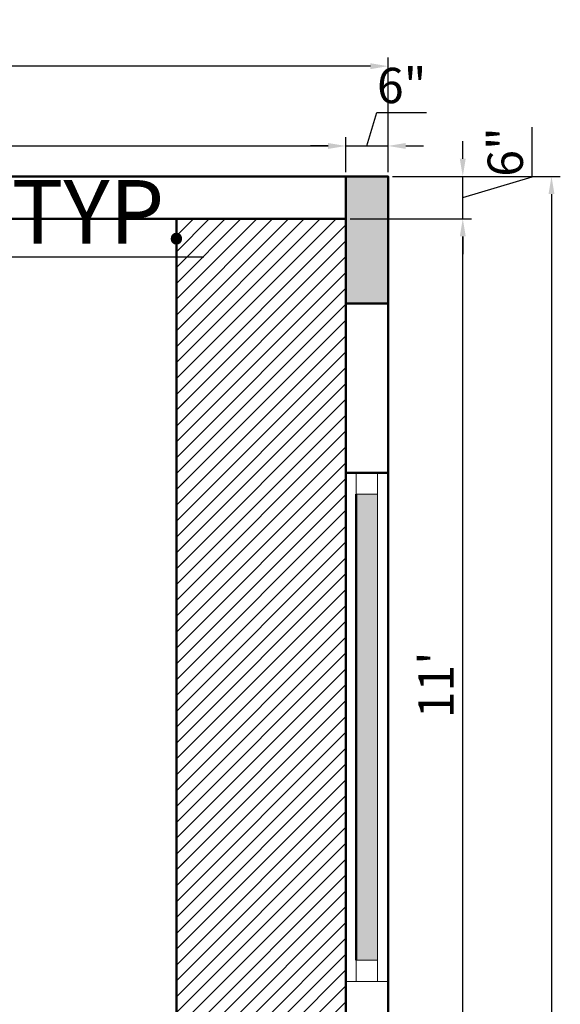
# Model space of a CAD drawing. Units: inches. Extents: x 3064 to 19385, y 846 to 15425.
# Tile 48 of 108: x 5481 to 5557, y 1275 to 1414. Entities that reach past the tile are written whole.
import ezdxf

# ---------------------------------------------------------------- set-up
doc = ezdxf.new("R2010")
doc.units = ezdxf.units.IN
for name, color, linetype, lineweight in [('A-ANNO-DIMS', 2, 'Continuous', 18), ('A-COLS', 1, 'Continuous', 35), ('A-FURN-PATT', 252, 'Continuous', 13), ('A-GLAZ', 4, 'Continuous', 18), ('A-WALL', 7, 'Continuous', 50)]:
    doc.layers.add(name, color=color, linetype=linetype, lineweight=lineweight)
doc.styles.get("Standard").update_dxf_attribs({"font": 'arial.ttf'})
doc.dimstyles.new('ISO-25', dxfattribs={"dimtxt": 9, "dimasz": 2.5, "dimexe": 1.25, "dimexo": 0.625, "dimtad": 1, "dimdec": 1, "dimlunit": 3, "dimtxsty": 'Standard', "dimcen": 2.5, "dimadec": 0, "dimazin": 0, "dimtfac": 1, "dimtdec": 1, "dimtmove": 0, "dimatfit": 3, "dimfxl": 1, "dimarcsym": 0})

# ---------------------------------------------------------------- blocks, each defined once
blk = doc.blocks.new('*D86')
at = {"layer": 'A-ANNO-DIMS', "color": 0, "lineweight": -2, "transparency": 16777216}
for p, q in [((5527.64, 1386.1), (5544.85, 1386.1)), ((5543.6, 1256.6), (5543.6, 1383.6)), ((5533.64, 1254.1), (5544.85, 1254.1))]:
    blk.add_line(p, q, dxfattribs=at)
at = {"layer": 'A-ANNO-DIMS', "color": 0, "transparency": 16777216}
for points in [[(5543.18, 1383.6), (5544.02, 1383.6), (5543.6, 1386.1)], [(5543.18, 1256.6), (5544.02, 1256.6), (5543.6, 1254.1)]]:
    blk.add_solid(points, dxfattribs=at)
at = {"layer": 'Defpoints', "color": 0, "transparency": 16777216}
for p in [(5527.02, 1386.1), (5543.6, 1386.1), (5533.02, 1254.1)]:
    blk.add_point(p, dxfattribs=at)
at = {"layer": 'A-ANNO-DIMS', "color": 0, "transparency": 16777216, "insert": (5540.46, 1320.1), "char_height": 5, "attachment_point": 5, "rotation": 90}
blk.add_mtext("11'", dxfattribs=at)
blk = doc.blocks.new('*D87')
at = {"layer": 'A-ANNO-DIMS', "color": 0, "lineweight": -2, "transparency": 16777216}
for p, q in [((5553.45, 1392.05), (5553.45, 1399.07)), ((5543.6, 1394.6), (5543.6, 1397.1)), ((5533.64, 1392.1), (5544.85, 1392.1)), ((5543.6, 1386.1), (5543.6, 1392.1)), ((5543.6, 1386.1), (5543.6, 1392.1)), ((5543.6, 1389.1), (5553.45, 1392.05)), ((5527.64, 1386.1), (5544.85, 1386.1)), ((5543.6, 1383.6), (5543.6, 1381.1))]:
    blk.add_line(p, q, dxfattribs=at)
at = {"layer": 'A-ANNO-DIMS', "color": 0, "transparency": 16777216}
for points in [[(5543.18, 1394.6), (5544.02, 1394.6), (5543.6, 1392.1)], [(5543.18, 1383.6), (5544.02, 1383.6), (5543.6, 1386.1)]]:
    blk.add_solid(points, dxfattribs=at)
at = {"layer": 'Defpoints', "color": 0, "transparency": 16777216}
for p in [(5533.02, 1392.1), (5543.6, 1392.1), (5527.02, 1386.1)]:
    blk.add_point(p, dxfattribs=at)
at = {"layer": 'A-ANNO-DIMS', "color": 0, "transparency": 16777216, "insert": (5550.27, 1395.56), "char_height": 5, "attachment_point": 5, "rotation": 90}
blk.add_mtext('6"', dxfattribs=at)
blk = doc.blocks.new('*D88')
at = {"layer": 'A-ANNO-DIMS', "color": 0, "lineweight": -2, "transparency": 16777216}
for p, q in [((5533.64, 1392.1), (5557.42, 1392.1)), ((5556.17, 1389.6), (5556.17, 902.6)), ((5533.64, 900.1), (5557.42, 900.1))]:
    blk.add_line(p, q, dxfattribs=at)
at = {"layer": 'A-ANNO-DIMS', "color": 0, "transparency": 16777216}
for points in [[(5555.75, 1389.6), (5556.59, 1389.6), (5556.17, 1392.1)], [(5555.75, 902.6), (5556.59, 902.6), (5556.17, 900.1)]]:
    blk.add_solid(points, dxfattribs=at)
at = {"layer": 'Defpoints', "color": 0, "transparency": 16777216}
for p in [(5533.02, 1392.1), (5533.02, 900.1), (5556.17, 900.1)]:
    blk.add_point(p, dxfattribs=at)
at = {"layer": 'A-ANNO-DIMS', "color": 0, "transparency": 16777216, "insert": (5553.04, 1146.1), "char_height": 5, "attachment_point": 5, "rotation": 90}
blk.add_mtext("41'", dxfattribs=at)
blk = doc.blocks.new('*D92')
at = {"layer": 'A-ANNO-DIMS', "color": 0, "lineweight": -2, "transparency": 16777216}
for p, q in [((5332.02, 1392.72), (5332.02, 1397.66)), ((5527.02, 1392.72), (5527.02, 1397.66)), ((5334.52, 1396.41), (5524.52, 1396.41))]:
    blk.add_line(p, q, dxfattribs=at)
at = {"layer": 'A-ANNO-DIMS', "color": 0, "transparency": 16777216}
for points in [[(5334.52, 1396.83), (5334.52, 1395.99), (5332.02, 1396.41)], [(5524.52, 1396.83), (5524.52, 1395.99), (5527.02, 1396.41)]]:
    blk.add_solid(points, dxfattribs=at)
at = {"layer": 'Defpoints', "color": 0, "transparency": 16777216}
for p in [(5527.02, 1396.41), (5332.02, 1392.1), (5527.02, 1392.1)]:
    blk.add_point(p, dxfattribs=at)
at = {"layer": 'A-ANNO-DIMS', "color": 0, "transparency": 16777216, "insert": (5429.52, 1399.59), "char_height": 5, "attachment_point": 5}
blk.add_mtext('16\'-3"', dxfattribs=at)
blk = doc.blocks.new('*D93')
at = {"layer": 'A-ANNO-DIMS', "color": 0, "lineweight": -2, "transparency": 16777216}
for p, q in [((5530.02, 1396.41), (5531.44, 1401.15)), ((5531.44, 1401.15), (5538.46, 1401.15)), ((5527.02, 1392.72), (5527.02, 1397.66)), ((5533.02, 1392.72), (5533.02, 1397.66)), ((5524.52, 1396.41), (5522.02, 1396.41)), ((5527.02, 1396.41), (5533.02, 1396.41)), ((5527.02, 1396.41), (5533.02, 1396.41)), ((5535.52, 1396.41), (5538.02, 1396.41))]:
    blk.add_line(p, q, dxfattribs=at)
at = {"layer": 'A-ANNO-DIMS', "color": 0, "transparency": 16777216}
for points in [[(5524.52, 1396.83), (5524.52, 1395.99), (5527.02, 1396.41)], [(5535.52, 1396.83), (5535.52, 1395.99), (5533.02, 1396.41)]]:
    blk.add_solid(points, dxfattribs=at)
at = {"layer": 'Defpoints', "color": 0, "transparency": 16777216}
for p in [(5533.02, 1396.41), (5527.02, 1392.1), (5533.02, 1392.1)]:
    blk.add_point(p, dxfattribs=at)
at = {"layer": 'A-ANNO-DIMS', "color": 0, "transparency": 16777216, "insert": (5534.95, 1404.33), "char_height": 5, "attachment_point": 5}
blk.add_mtext('6"', dxfattribs=at)
blk = doc.blocks.new('*D94')
at = {"layer": 'A-ANNO-DIMS', "color": 0, "lineweight": -2, "transparency": 16777216}
for p, q in [((5191.02, 1392.72), (5191.02, 1408.96)), ((5533.02, 1392.72), (5533.02, 1408.96)), ((5530.52, 1407.71), (5193.52, 1407.71))]:
    blk.add_line(p, q, dxfattribs=at)
at = {"layer": 'A-ANNO-DIMS', "color": 0, "transparency": 16777216}
for points in [[(5193.52, 1408.12), (5193.52, 1407.29), (5191.02, 1407.71)], [(5530.52, 1408.12), (5530.52, 1407.29), (5533.02, 1407.71)]]:
    blk.add_solid(points, dxfattribs=at)
at = {"layer": 'Defpoints', "color": 0, "transparency": 16777216}
for p in [(5191.02, 1407.71), (5191.02, 1392.1), (5533.02, 1392.1)]:
    blk.add_point(p, dxfattribs=at)
at = {"layer": 'A-ANNO-DIMS', "color": 0, "transparency": 16777216, "insert": (5362.02, 1410.88), "char_height": 5, "attachment_point": 5}
blk.add_mtext('28\'-6"', dxfattribs=at)
blk = doc.blocks.new('WIN-1900')
blk.add_line((3, 0), (3, 66))
blk.add_lwpolyline([(3, 66), (0, 66), (0, 69), (3, 69)], close=True)
blk = doc.blocks.new('*D443')
at = {"layer": 'A-ANNO-DIMS', "color": 0, "lineweight": -2, "transparency": 16777216}
for p, q in [((5356.02, 1385.47), (5356.02, 1379.45)), ((5392.02, 1385.47), (5392.02, 1379.45)), ((5358.52, 1380.7), (5389.52, 1380.7)), ((5392.02, 1380.7), (5506.9, 1380.7))]:
    blk.add_line(p, q, dxfattribs=at)
at = {"layer": 'A-ANNO-DIMS', "color": 0, "transparency": 16777216}
for points in [[(5358.52, 1381.11), (5358.52, 1380.28), (5356.02, 1380.7)], [(5389.52, 1381.11), (5389.52, 1380.28), (5392.02, 1380.7)]]:
    blk.add_solid(points, dxfattribs=at)
at = {"layer": 'Defpoints', "color": 0, "transparency": 16777216}
for p in [(5356.02, 1386.1), (5392.02, 1386.1), (5392.02, 1380.7)]:
    blk.add_point(p, dxfattribs=at)
at = {"layer": 'A-ANNO-DIMS', "color": 0, "transparency": 16777216, "insert": (5450.71, 1385.92), "char_height": 9, "attachment_point": 5}
blk.add_mtext('W1000-B 3\'-0" TYP.', dxfattribs=at)

msp = doc.modelspace()

# ---------------------------------------------------------------- hatches: boundary and pattern name
at = {"layer": 'A-COLS'}
h = msp.add_hatch(color=256, dxfattribs=at)
h.dxf.hatch_style = 1
h.paths.add_polyline_path([(5533.02, 1374.1), (5533.02, 1392.1), (5527.02, 1392.1), (5527.02, 1374.1)])
at = {"layer": 'A-FURN-PATT'}
h = msp.add_hatch(dxfattribs=at)
h.set_pattern_fill('ANSI31', color=256, scale=0.5)
h.set_pattern_definition([(45, (848.524, -4.2436), (-1.122532, 1.122532), [])])
h.paths.add_polyline_path([(5503.02, 1254.1), (5527.02, 1254.1), (5527.02, 1386.1), (5503.02, 1386.1)])
at = {"layer": 'A-GLAZ'}
h = msp.add_hatch(color=256, dxfattribs=at)
h.dxf.hatch_style = 1
h.paths.add_polyline_path([(5528.52, 1281.1), (5531.52, 1281.1), (5531.52, 1347.1), (5528.52, 1347.1)])

# ---------------------------------------------------------------- linework, layer by layer
msp.add_line((5533.02, 1278.1), (5527.02, 1278.1), dxfattribs=at)
msp.add_lwpolyline([(5531.52, 1278.1), (5528.52, 1278.1), (5528.52, 1281.1), (5531.52, 1281.1)], close=True, dxfattribs=at)
at = {"layer": 'A-WALL'}
for p, q in [((5533.02, 1392.1), (5191.02, 1392.1)), ((5533.02, 900.1), (5533.02, 1392.1)), ((5527.02, 1386.1), (5332.02, 1386.1)), ((5503.02, 1254.1), (5503.02, 1386.1)), ((5527.02, 1254.1), (5527.02, 1386.1)), ((5527.02, 1350.1), (5533.02, 1350.1)), ((5528.52, 1347.1), (5528.52, 1281.1))]:
    msp.add_line(p, q, dxfattribs=at)
msp.add_lwpolyline([(5533.02, 1374.1), (5533.02, 1392.1), (5527.02, 1392.1), (5527.02, 1374.1)], close=True, dxfattribs=at)

# ---------------------------------------------------------------- block references
at = {"layer": 'A-GLAZ'}
msp.add_blockref('WIN-1900', (5528.52, 1281.1), dxfattribs=at)

# ---------------------------------------------------------------- dimensions: what is measured, and where the dimension line sits
at = {"layer": 'A-ANNO-DIMS'}
for base, p1, p2, override, picture, middle in [((5191.02, 1407.71), (5533.02, 1392.1), (5191.02, 1392.1), {"dimtxt": 5, "dimclrd": 0, "dimclre": 0, "dimclrt": 0}, '*D94', (5362.02, 1410.88)), ((5533.02, 1396.41), (5527.02, 1392.1), (5533.02, 1392.1), {"dimtxt": 5, "dimclrd": 0, "dimclre": 0, "dimclrt": 0, "dimtmove": 1}, '*D93', (5532.06, 1404.33)), ((5527.02, 1396.41), (5332.02, 1392.1), (5527.02, 1392.1), {"dimtxt": 5, "dimclrd": 0, "dimclre": 0, "dimclrt": 0, "dimtmove": 1}, '*D92', (5429.52, 1399.59))]:
    dim = msp.add_linear_dim(base=base, p1=p1, p2=p2, dimstyle='ISO-25', override=override, dxfattribs=at)
    dim.commit()
    dim.dimension.update_dxf_attribs({"geometry": picture, "text_midpoint": middle})
dim = msp.add_linear_dim(base=(5392.02, 1380.7), p1=(5356.02, 1386.1), p2=(5392.02, 1386.1), text='W1000-B <> TYP.', dimstyle='ISO-25', override={"dimdec": 1, "dimrnd": 0, "dimzin": 1, "dimlunit": 4, "dimfrac": 2}, dxfattribs=at)
dim.commit()
dim.dimension.update_dxf_attribs({"geometry": '*D443', "text_midpoint": (5450.71, 1385.92)})
for base, p1, p2, override, picture, middle in [((5543.6, 1392.1), (5527.02, 1386.1), (5533.02, 1392.1), {"dimtxt": 5, "dimclrd": 0, "dimclre": 0, "dimclrt": 0, "dimtmove": 1}, '*D87', (5550.27, 1392.68)), ((5556.17, 900.1), (5533.02, 1392.1), (5533.02, 900.1), {"dimtxt": 5, "dimclrd": 0, "dimclre": 0, "dimclrt": 0}, '*D88', (5553.04, 1146.1)), ((5543.6, 1386.1), (5533.02, 1254.1), (5527.02, 1386.1), {"dimtxt": 5, "dimclrd": 0, "dimclre": 0, "dimclrt": 0, "dimtmove": 1}, '*D86', (5540.46, 1320.1))]:
    dim = msp.add_linear_dim(base=base, p1=p1, p2=p2, angle=90, dimstyle='ISO-25', override=override, dxfattribs=at)
    dim.commit()
    dim.dimension.update_dxf_attribs({"geometry": picture, "text_midpoint": middle})

doc.saveas('drawing.dxf')
